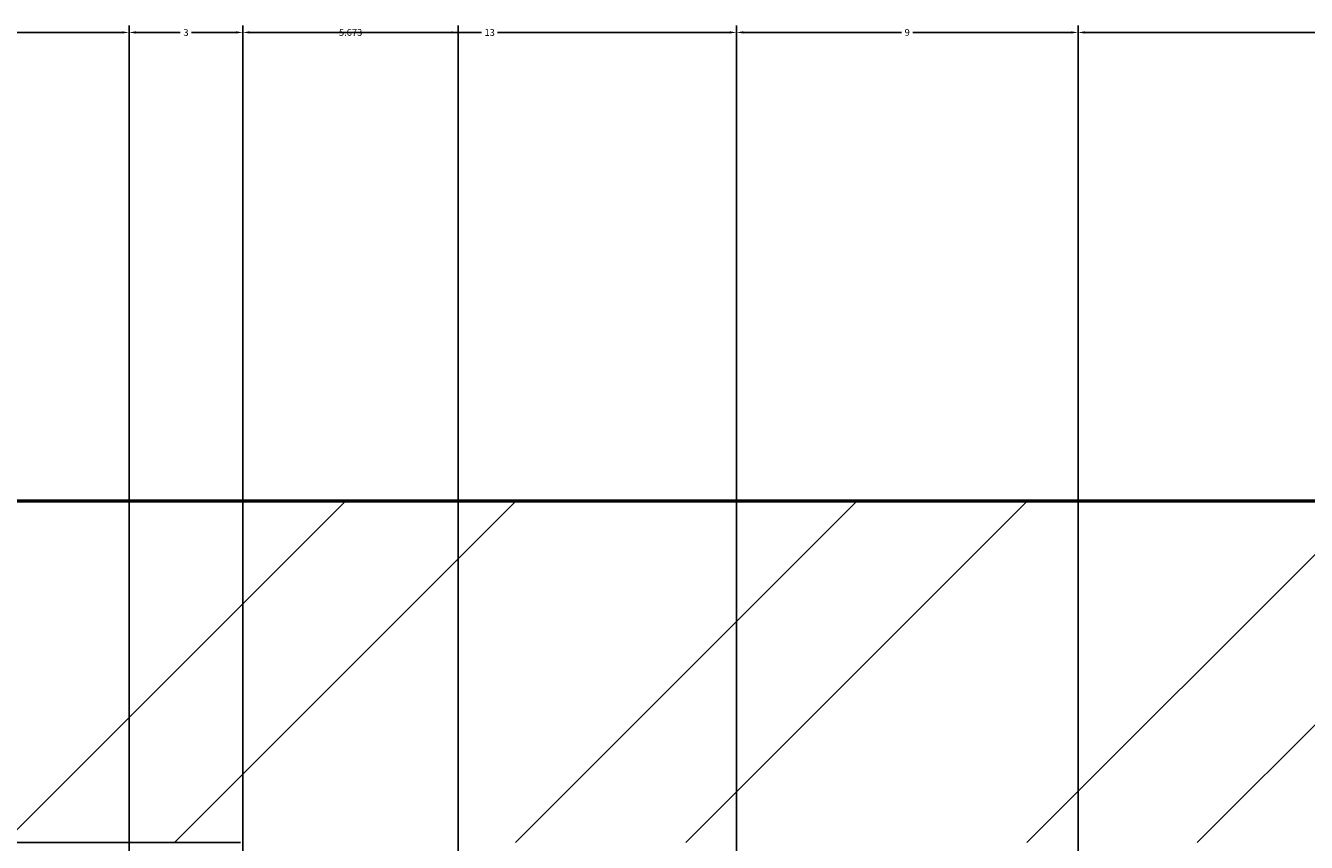
# Model space of a CAD drawing. Units: inches. Extents: x 2812 to 3051, y 1398 to 1659.
# Tile 55 of 65: x 2878 to 2911, y 1638 to 1659. Entities that reach past the tile are written whole.
import ezdxf

# ---------------------------------------------------------------- set-up
doc = ezdxf.new("R2010")
doc.units = ezdxf.units.IN
for name, color, linetype, lineweight in [('A-ANNO-DIMS', 2, 'Continuous', 18), ('S-CONC', 7, 'Continuous', 50), ('S-CONC-PATT', 8, 'Continuous', 18)]:
    doc.layers.add(name, color=color, linetype=linetype, lineweight=lineweight)
doc.styles.get("Standard").update_dxf_attribs({"font": 'arial.ttf'})
doc.dimstyles.get("Standard").update_dxf_attribs({"dimtxt": 0.18, "dimasz": 0.18, "dimexe": 0.18, "dimexo": 0.0625, "dimgap": 0.09, "dimtad": 0, "dimtih": 1, "dimtoh": 1, "dimdec": 4, "dimzin": 0, "dimdsep": 46, "dimtxsty": 'Standard', "dimcen": 0.09, "dimadec": 0, "dimazin": 0, "dimtfac": 1, "dimtdec": 4, "dimtofl": 0, "dimtmove": 0, "dimatfit": 3, "dimfxl": 1, "dimtolj": 1, "dimtzin": 0, "dimarcsym": 0})

# ---------------------------------------------------------------- blocks, each defined once
blk = doc.blocks.new('*D15')
at = {"layer": 'A-ANNO-DIMS', "color": 0, "lineweight": -2, "transparency": 16777216}
for p, q in [((2844.385, 1637.882), (2844.385, 1659.35)), ((2880.385, 1637.882), (2880.385, 1659.35)), ((2844.565, 1659.17), (2862.166, 1659.17)), ((2880.205, 1659.17), (2862.604, 1659.17))]:
    blk.add_line(p, q, dxfattribs=at)
at = {"layer": 'A-ANNO-DIMS', "color": 0, "transparency": 16777216}
for points in [[(2844.565, 1659.2), (2844.565, 1659.14), (2844.385, 1659.17)], [(2880.205, 1659.2), (2880.205, 1659.14), (2880.385, 1659.17)]]:
    blk.add_solid(points, dxfattribs=at)
at = {"layer": 'Defpoints', "color": 0, "transparency": 16777216}
for p in [(2880.385, 1659.17), (2844.385, 1637.82), (2880.385, 1637.82)]:
    blk.add_point(p, dxfattribs=at)
at = {"layer": 'A-ANNO-DIMS', "color": 0, "transparency": 16777216, "insert": (2862.385, 1659.17), "char_height": 0.18, "attachment_point": 5}
blk.add_mtext('\\A1;36', dxfattribs=at)
blk = doc.blocks.new('*D16')
at = {"layer": 'A-ANNO-DIMS', "color": 0, "lineweight": -2, "transparency": 16777216}
for p, q in [((2880.385, 1637.882), (2880.385, 1659.35)), ((2883.385, 1637.882), (2883.385, 1659.35)), ((2880.565, 1659.17), (2881.736, 1659.17)), ((2883.205, 1659.17), (2882.034, 1659.17))]:
    blk.add_line(p, q, dxfattribs=at)
at = {"layer": 'A-ANNO-DIMS', "color": 0, "transparency": 16777216}
for points in [[(2880.565, 1659.2), (2880.565, 1659.14), (2880.385, 1659.17)], [(2883.205, 1659.2), (2883.205, 1659.14), (2883.385, 1659.17)]]:
    blk.add_solid(points, dxfattribs=at)
at = {"layer": 'Defpoints', "color": 0, "transparency": 16777216}
for p in [(2883.385, 1659.17), (2880.385, 1637.82), (2883.385, 1637.82)]:
    blk.add_point(p, dxfattribs=at)
at = {"layer": 'A-ANNO-DIMS', "color": 0, "transparency": 16777216, "insert": (2881.885, 1659.17), "char_height": 0.18, "attachment_point": 5}
blk.add_mtext('\\A1;3', dxfattribs=at)
blk = doc.blocks.new('*D17')
at = {"layer": 'A-ANNO-DIMS', "color": 0, "lineweight": -2, "transparency": 16777216}
for p, q in [((2883.385, 1637.882), (2883.385, 1659.35)), ((2896.385, 1625.882), (2896.385, 1659.35)), ((2883.565, 1659.17), (2889.674, 1659.17)), ((2896.205, 1659.17), (2890.095, 1659.17))]:
    blk.add_line(p, q, dxfattribs=at)
at = {"layer": 'A-ANNO-DIMS', "color": 0, "transparency": 16777216}
for points in [[(2883.565, 1659.2), (2883.565, 1659.14), (2883.385, 1659.17)], [(2896.205, 1659.2), (2896.205, 1659.14), (2896.385, 1659.17)]]:
    blk.add_solid(points, dxfattribs=at)
at = {"layer": 'Defpoints', "color": 0, "transparency": 16777216}
for p in [(2896.385, 1659.17), (2883.385, 1637.82), (2896.385, 1625.82)]:
    blk.add_point(p, dxfattribs=at)
at = {"layer": 'A-ANNO-DIMS', "color": 0, "transparency": 16777216, "insert": (2889.885, 1659.17), "char_height": 0.18, "attachment_point": 5}
blk.add_mtext('\\A1;13', dxfattribs=at)
blk = doc.blocks.new('*D18')
at = {"layer": 'A-ANNO-DIMS', "color": 0, "lineweight": -2, "transparency": 16777216}
for p, q in [((2896.385, 1625.882), (2896.385, 1659.35)), ((2905.385, 1625.882), (2905.385, 1659.35)), ((2896.565, 1659.17), (2900.736, 1659.17)), ((2905.205, 1659.17), (2901.034, 1659.17))]:
    blk.add_line(p, q, dxfattribs=at)
at = {"layer": 'A-ANNO-DIMS', "color": 0, "transparency": 16777216}
for points in [[(2896.565, 1659.2), (2896.565, 1659.14), (2896.385, 1659.17)], [(2905.205, 1659.2), (2905.205, 1659.14), (2905.385, 1659.17)]]:
    blk.add_solid(points, dxfattribs=at)
at = {"layer": 'Defpoints', "color": 0, "transparency": 16777216}
for p in [(2905.385, 1659.17), (2896.385, 1625.82), (2905.385, 1625.82)]:
    blk.add_point(p, dxfattribs=at)
at = {"layer": 'A-ANNO-DIMS', "color": 0, "transparency": 16777216, "insert": (2900.885, 1659.17), "char_height": 0.18, "attachment_point": 5}
blk.add_mtext('\\A1;9', dxfattribs=at)
blk = doc.blocks.new('*D19')
at = {"layer": 'A-ANNO-DIMS', "color": 0, "lineweight": -2, "transparency": 16777216}
for p, q in [((2905.385, 1625.882), (2905.385, 1659.35)), ((2941.385, 1625.882), (2941.385, 1659.35)), ((2905.565, 1659.17), (2923.166, 1659.17)), ((2941.205, 1659.17), (2923.604, 1659.17))]:
    blk.add_line(p, q, dxfattribs=at)
at = {"layer": 'A-ANNO-DIMS', "color": 0, "transparency": 16777216}
for points in [[(2905.565, 1659.2), (2905.565, 1659.14), (2905.385, 1659.17)], [(2941.205, 1659.2), (2941.205, 1659.14), (2941.385, 1659.17)]]:
    blk.add_solid(points, dxfattribs=at)
at = {"layer": 'Defpoints', "color": 0, "transparency": 16777216}
for p in [(2941.385, 1659.17), (2905.385, 1625.82), (2941.385, 1625.82)]:
    blk.add_point(p, dxfattribs=at)
at = {"layer": 'A-ANNO-DIMS', "color": 0, "transparency": 16777216, "insert": (2923.385, 1659.17), "char_height": 0.18, "attachment_point": 5}
blk.add_mtext('\\A1;36', dxfattribs=at)
blk = doc.blocks.new('*D39')
at = {"layer": 'A-ANNO-DIMS', "color": 0, "lineweight": -2, "transparency": 16777216}
for p, q in [((2883.322, 1637.82), (2811.806, 1637.82)), ((2811.986, 1637.64), (2811.986, 1632)), ((2811.986, 1626), (2811.986, 1631.64)), ((2896.322, 1625.82), (2811.806, 1625.82))]:
    blk.add_line(p, q, dxfattribs=at)
at = {"layer": 'A-ANNO-DIMS', "color": 0, "transparency": 16777216}
for points in [[(2811.956, 1637.64), (2812.016, 1637.64), (2811.986, 1637.82)], [(2811.956, 1626), (2812.016, 1626), (2811.986, 1625.82)]]:
    blk.add_solid(points, dxfattribs=at)
at = {"layer": 'Defpoints', "color": 0, "transparency": 16777216}
for p in [(2811.986, 1637.82), (2883.385, 1637.82), (2896.385, 1625.82)]:
    blk.add_point(p, dxfattribs=at)
at = {"layer": 'A-ANNO-DIMS', "color": 0, "transparency": 16777216, "insert": (2811.986, 1631.82), "char_height": 0.18, "attachment_point": 5}
blk.add_mtext('\\A1;12', dxfattribs=at)
blk = doc.blocks.new('*D58')
at = {"layer": 'A-ANNO-DIMS', "color": 0, "lineweight": -2, "transparency": 16777216}
for p, q in [((2880.385, 1472.098), (2880.385, 1659.35)), ((2883.385, 1472.098), (2883.385, 1659.35)), ((2880.565, 1659.17), (2881.736, 1659.17)), ((2883.205, 1659.17), (2882.034, 1659.17))]:
    blk.add_line(p, q, dxfattribs=at)
at = {"layer": 'A-ANNO-DIMS', "color": 0, "transparency": 16777216}
for points in [[(2880.565, 1659.2), (2880.565, 1659.14), (2880.385, 1659.17)], [(2883.205, 1659.2), (2883.205, 1659.14), (2883.385, 1659.17)]]:
    blk.add_solid(points, dxfattribs=at)
at = {"layer": 'Defpoints', "color": 0, "transparency": 16777216}
for p in [(2883.385, 1659.17), (2880.385, 1472.035), (2883.385, 1472.035)]:
    blk.add_point(p, dxfattribs=at)
at = {"layer": 'A-ANNO-DIMS', "color": 0, "transparency": 16777216, "insert": (2881.885, 1659.17), "char_height": 0.18, "attachment_point": 5}
blk.add_mtext('\\A1;3', dxfattribs=at)
blk = doc.blocks.new('*D59')
at = {"layer": 'A-ANNO-DIMS', "color": 0, "lineweight": -2, "transparency": 16777216}
for p, q in [((2883.385, 1452.098), (2883.385, 1659.35)), ((2889.058, 1467.465), (2889.058, 1659.35)), ((2883.565, 1659.17), (2885.828, 1659.17)), ((2888.878, 1659.17), (2886.615, 1659.17))]:
    blk.add_line(p, q, dxfattribs=at)
at = {"layer": 'A-ANNO-DIMS', "color": 0, "transparency": 16777216}
for points in [[(2883.565, 1659.2), (2883.565, 1659.14), (2883.385, 1659.17)], [(2888.878, 1659.2), (2888.878, 1659.14), (2889.058, 1659.17)]]:
    blk.add_solid(points, dxfattribs=at)
at = {"layer": 'Defpoints', "color": 0, "transparency": 16777216}
for p in [(2889.058, 1659.17), (2889.058, 1467.402), (2883.385, 1452.035)]:
    blk.add_point(p, dxfattribs=at)
at = {"layer": 'A-ANNO-DIMS', "color": 0, "transparency": 16777216, "insert": (2886.221, 1659.17), "char_height": 0.18, "attachment_point": 5}
blk.add_mtext('\\A1;5.673', dxfattribs=at)

msp = doc.modelspace()

# ---------------------------------------------------------------- hatches: boundary and pattern name
at = {"layer": 'S-CONC-PATT'}
h = msp.add_hatch(dxfattribs=at)
h.set_pattern_fill('ANSI32', color=256)
h.paths.add_polyline_path([(3027.3849, 1646.82), (2835.3849, 1646.82), (2835.3849, 1603.2296), (2844.3849, 1603.2296), (2844.3849, 1637.82), (3018.3849, 1637.82), (3018.3849, 1602.5441), (3027.3849, 1602.5441)])
h.paths.add_polyline_path([(2844.3849, 1594.2296), (2835.3849, 1594.2296), (2835.3849, 1550.82), (3027.3849, 1550.82), (3027.3849, 1593.5441), (3018.3849, 1593.5441), (3018.3849, 1559.82), (2844.3849, 1559.82)])
h.paths.add_polyline_path([(2844.3849, 1482.0354), (2835.3849, 1482.0354), (2835.3849, 1463.4959), (2844.3849, 1463.4959)])
h.paths.add_polyline_path([(2844.3849, 1461.4959), (2835.3849, 1461.4959), (2835.3849, 1416.0354), (2844.3849, 1416.0354)])
h.paths.add_polyline_path([(3027.3849, 1482.0354), (3018.3849, 1482.0354), (3018.3849, 1463.2854), (3027.3849, 1463.2854)])
h.paths.add_polyline_path([(3027.3849, 1461.2854), (3018.3849, 1461.2854), (3018.3849, 1416.0354), (3027.3849, 1416.0354)])
h.paths.add_polyline_path([(2961.3849, 1448.4738), (2952.3849, 1448.4738), (2952.3849, 1416.0354), (2961.3849, 1416.0354)])
h.paths.add_polyline_path([(2961.3849, 1462.3026), (2952.3849, 1462.3026), (2952.3849, 1450.4738), (2961.3849, 1450.4738)])
h.paths.add_polyline_path([(2961.3849, 1472.0354), (2952.3849, 1472.0354), (2952.3849, 1462.3026), (2961.3849, 1462.3026)])

# ---------------------------------------------------------------- linework, layer by layer
at = {"layer": 'S-CONC'}
msp.add_line((2835.3849, 1646.82), (3027.3849, 1646.82), dxfattribs=at)

# ---------------------------------------------------------------- dimensions: what is measured, and where the dimension line sits
at = {"layer": 'A-ANNO-DIMS'}
for base, p1, p2, override, picture, middle in [((2880.3849, 1659.17), (2844.3849, 1637.82), (2880.3849, 1637.82), {"dimdec": 0, "dimlfac": 1, "dimrnd": 0, "dimzin": 0, "dimdsep": 46, "dimlunit": 2}, '*D15', (2862.3849, 1659.17)), ((2883.3849, 1659.17), (2880.3849, 1637.82), (2883.3849, 1637.82), {"dimdec": 0, "dimlfac": 1, "dimrnd": 0, "dimzin": 0, "dimdsep": 46, "dimlunit": 2}, '*D16', (2881.8849, 1659.17)), ((2883.3849, 1659.17), (2880.3849, 1472.0354), (2883.3849, 1472.0354), {"dimdec": 0, "dimlfac": 1, "dimrnd": 0, "dimzin": 0, "dimdsep": 46, "dimlunit": 2}, '*D58', (2881.8849, 1659.17)), ((2896.3849, 1659.17), (2883.3849, 1637.82), (2896.3849, 1625.82), {"dimdec": 0, "dimlfac": 1, "dimrnd": 0, "dimzin": 0, "dimdsep": 46, "dimlunit": 2}, '*D17', (2889.8849, 1659.17)), ((2889.0577, 1659.17), (2883.3849, 1452.0354), (2889.0577, 1467.4024), {"dimdec": 3, "dimlfac": 1, "dimrnd": 0, "dimzin": 0, "dimdsep": 46, "dimlunit": 2}, '*D59', (2886.2213, 1659.17)), ((2905.3849, 1659.17), (2896.3849, 1625.82), (2905.3849, 1625.82), {"dimdec": 0, "dimlfac": 1, "dimrnd": 0, "dimzin": 0, "dimdsep": 46, "dimlunit": 2}, '*D18', (2900.8849, 1659.17)), ((2941.3849, 1659.17), (2905.3849, 1625.82), (2941.3849, 1625.82), {"dimdec": 0, "dimlfac": 1, "dimrnd": 0, "dimzin": 0, "dimdsep": 46, "dimlunit": 2}, '*D19', (2923.3849, 1659.17))]:
    dim = msp.add_linear_dim(base=base, p1=p1, p2=p2, dimstyle='Standard', override=override, dxfattribs=at)
    dim.commit()
    dim.dimension.update_dxf_attribs({"geometry": picture, "text_midpoint": middle})
dim = msp.add_linear_dim(base=(2811.9855, 1637.82), p1=(2896.3849, 1625.82), p2=(2883.3849, 1637.82), angle=90, dimstyle='Standard', override={"dimdec": 0, "dimlfac": 1, "dimrnd": 0, "dimzin": 0, "dimdsep": 46, "dimlunit": 2}, dxfattribs=at)
dim.commit()
dim.dimension.update_dxf_attribs({"geometry": '*D39', "text_midpoint": (2811.9855, 1631.82)})

doc.saveas('drawing.dxf')
